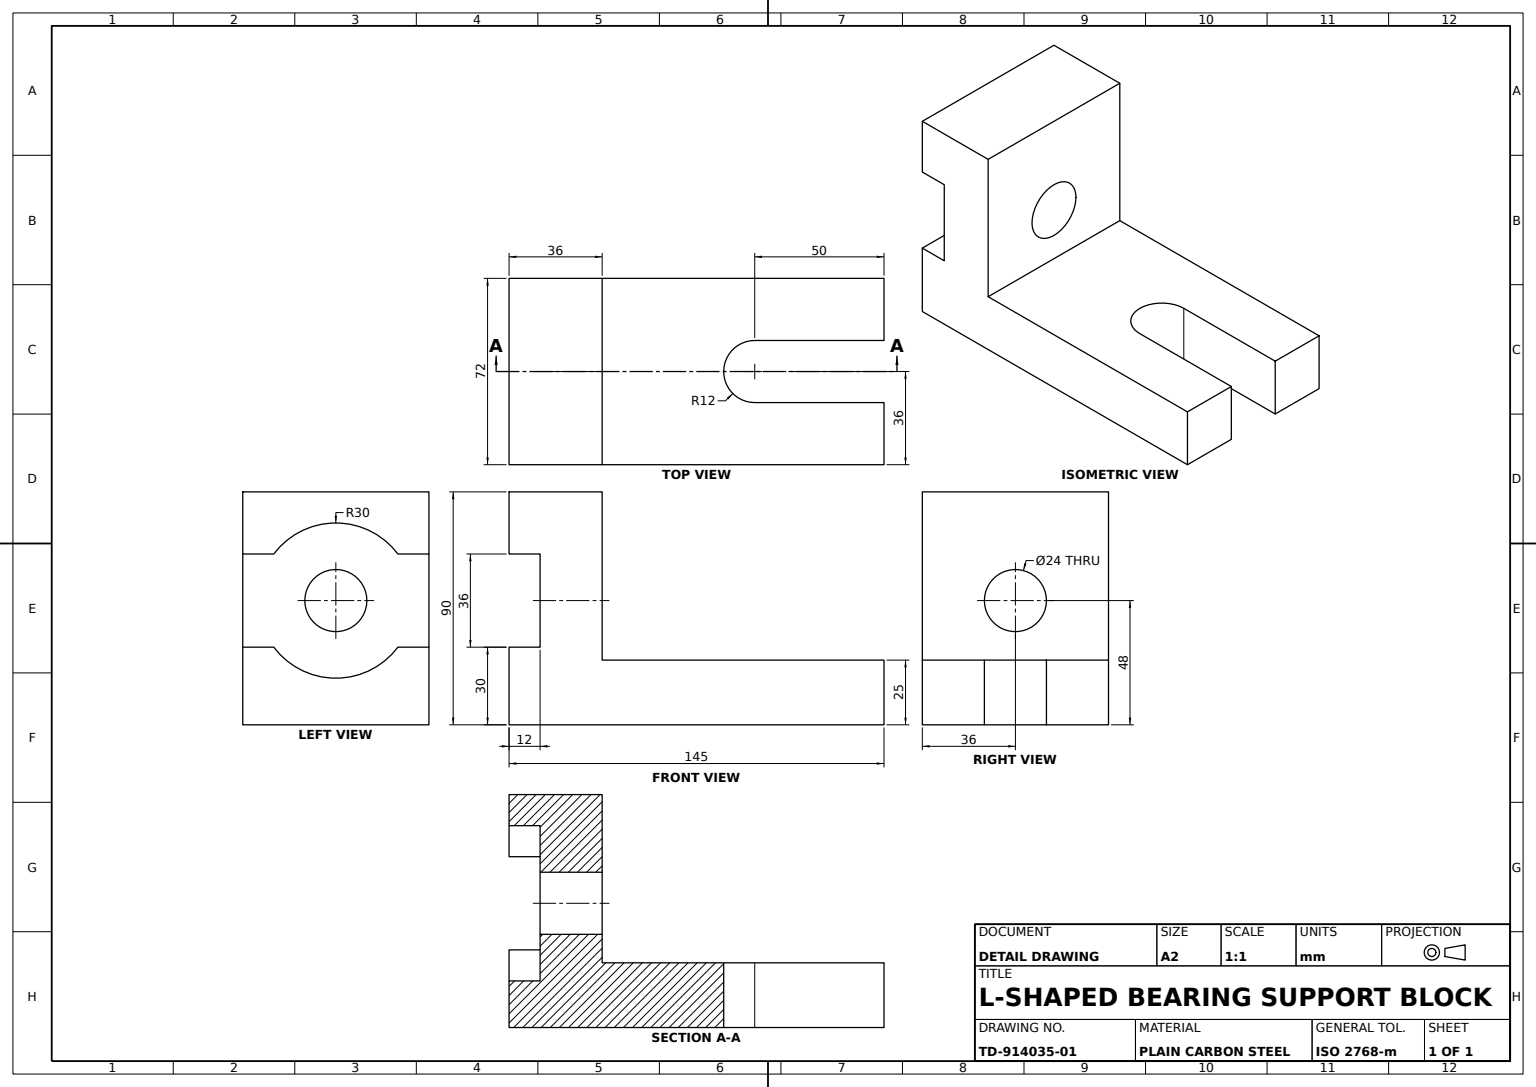
SolidWorks part; units mm, degrees
material "Plain Carbon Steel"
ref_plane "Front Plane" through (0, 0, 0) normal (0, 0, 1) x (1, 0, 0)
ref_plane "Top Plane" through (0, 0, 0) normal (0, 1, 0) x (1, 0, 0)
ref_plane "Right Plane" through (0, 0, 0) normal (1, 0, 0) x (0, 0, -1)
sketch "Base Plate Sketch" plane through (0, 0, 0) normal (0, 1, 0) x (1, 0, 0)
  line L1 (36, 0) -> (36, 72.5)
  line L2 (36, 72.5) -> (-36, 72.5)
  line L3 (-36, 72.5) -> (-36, -72.5)
  line L4 (-36, -72.5) -> (36, -72.5)
  line L5 (36, -72.5) -> (36, 0)
  dimension "D1" = 72
  dimension "D2" = 145
  dimension "D3" = 36
extrude "Base Plate" add sketch "Base Plate Sketch" along normal blind 25
sketch "Base Slot Sketch" plane through (0, 25, 0) normal (0, 1, 0) x (1, 0, 0)
  line L0 (36, -72.5) -> (36, 72.5) construction
  line L1 (36, 72.5) -> (-36, 72.5) construction
  line L2 (12, 22.5) -> (12, 72.5)
  line L3 (-12, 22.5) -> (-12, 72.5)
  line L4 (-12, 72.5) -> (12, 72.5)
  arc A0 (-12, 22.5) -> (12, 22.5) centre (0, 22.5) ccw
  dimension "D1" = 12
  dimension "D2" = 36
  dimension "D3" = 50
extrude "Base Slot" cut sketch "Base Slot Sketch" against normal blind 50
sketch "Upright Block Sketch" plane through (0, 25, 0) normal (0, 1, 0) x (1, 0, 0)
  line L0 (36, -72.5) -> (36, -36.5)
  line L1 (36, -72.5) -> (36, 72.5) construction
  line L2 (36, -36.5) -> (-36, -36.5)
  line L3 (-36, 72.5) -> (-36, -72.5) construction
  line L4 (-36, -36.5) -> (-36, -72.5)
  line L5 (-36, -72.5) -> (36, -72.5)
  dimension "D1" = 109
extrude "Upright Block" add sketch "Upright Block Sketch" along normal blind 65
sketch "Bearing Seat Sketch" plane through (0, 0, 72.5) normal (0, 0, 1) x (1, 0, 0)
  line L0 (-36, 0) -> (-36, 30)
  line L1 (-36, 90) -> (-36, 0) construction
  line L2 (-36, 30) -> (-24, 30)
  line L3 (36, 90) -> (36, 0) construction
  line L4 (36, 30) -> (36, 0)
  line L5 (36, 0) -> (-36, 0)
  line L6 (24, 30) -> (36, 30)
  line L7 (36, 90) -> (36, 66)
  line L8 (36, 66) -> (24, 66)
  line L9 (-36, 66) -> (-36, 90)
  line L10 (-36, 90) -> (36, 90)
  line L11 (-24, 66) -> (-36, 66)
  line L12 (36, 66) -> (36, 30)
  line L13 (-36, 66) -> (-36, 30)
  arc A0 (24, 66) -> (-24, 66) centre (0, 48) ccw
  arc A1 (-24, 30) -> (24, 30) centre (0, 48) ccw
  line M8 (36, 0) -> (36, 90)
  line M10 (-36, 90) -> (-36, 0)
  dimension "D1" = 30
  dimension "D2" = 12
extrude "Bearing Seat Cut" cut sketch "Bearing Seat Sketch" against normal blind 12 contours L2 A1 L6 L8 A0 L11 M8 M10
sketch "Through Bore Sketch" plane through (0, 0, 60.5) normal (0, 0, 1) x (1, 0, 0)
  line L0 (36, 30) -> (36, 66) construction
  line L1 (24, 30) -> (36, 30) construction
  circle A0 centre (0, 48) radius 12
  dimension "D1" = 24
  dimension "D2" = 36
  dimension "D3" = 18
extrude "Through Bore" cut sketch "Through Bore Sketch" against normal blind 106
